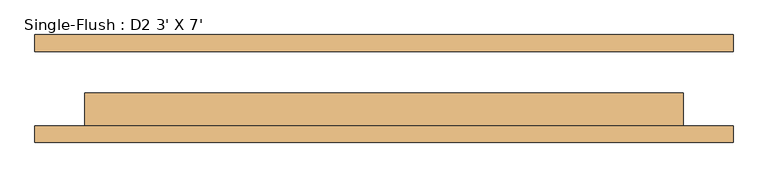
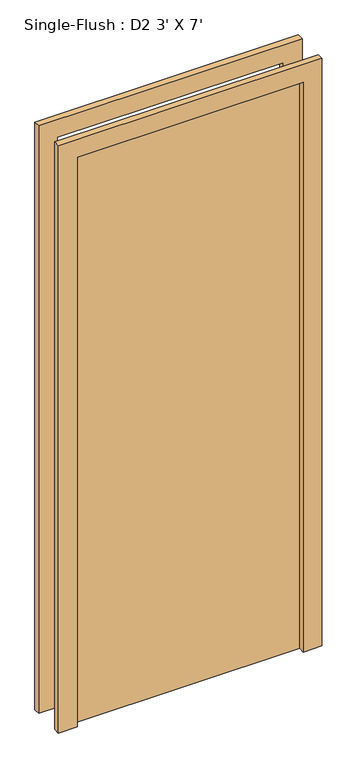
"""IFC4 building model written with IfcOpenShell, lengths in millimetres: door geometry, Single-Flush : D2 3' X 7'."""

from ifc_helpers import new_model, si_unit, frame, origin, origin_with_axes, place, context, project, spatial, polyline, outline, extrude, source, transform, mapped, element, save


def single_flush_d2_3_x_7_58d0fc15(model_context):
    return source(origin(), model_context, "Body", "SweptSolid", [
        extrude(outline(polyline([(2514.6, -533.4), (0.0, -533.4), (0.0, -457.2), (2438.4, -457.2), (2438.4, 457.2), (0.0, 457.2), (0.0, 533.4), (2514.6, 533.4), (2514.6, -533.4)])), frame((0.0, -82.55, 0.0), z_axis=(0.0, 1.0, 0.0), x_axis=(0.0, 0.0, 1.0)), (0.0, 0.0, 1.0), 25.4),
        extrude(outline(polyline([(2514.6, 533.4), (2514.6, -533.4), (0.0, -533.4), (0.0, -457.2), (2438.4, -457.2), (2438.4, 457.2), (0.0, 457.2), (0.0, 533.4), (2514.6, 533.4)])), frame((0.0, 57.15, 0.0), z_axis=(0.0, 1.0, 0.0), x_axis=(0.0, 0.0, 1.0)), (0.0, 0.0, 1.0), 25.4),
        extrude(outline(polyline([(457.2, -6.35), (457.2, -57.15), (-457.2, -57.15), (-457.2, -6.35), (457.2, -6.35)])), origin_with_axes(), (0.0, 0.0, 1.0), 2438.4),
    ])


if __name__ == "__main__":
    model = new_model("IFC4")
    model_context = context("Model", 3, world=origin())
    ifc_project = project(units=[si_unit("LENGTHUNIT", "METRE", prefix="MILLI")], contexts=[model_context])
    site = spatial("IfcSite", under=ifc_project)
    building = spatial("IfcBuilding", under=site)
    placement = place(None, origin())
    single_flush_d2_3_x_7_shape = single_flush_d2_3_x_7_58d0fc15(model_context)
    element("IfcDoor", 1, ObjectType="Single-Flush : D2 3' X 7'", at=placement, inside=building, context=model_context, shape_type="MappedRepresentation", body=[
        mapped(single_flush_d2_3_x_7_shape, transform((0.0, 0.0, 0.0), x_axis=(1.0, 0.0, 0.0), y_axis=(0.0, 1.0, 0.0), z_axis=(0.0, 0.0, 1.0))),
    ])
    save(model, "model.ifc")

# Revit data of these elements
# Type "Single-Flush : D2 3' X 7'"
#   Type Mark = "10"
#   Construction Type Id = "MDOOR"
#   Assembly Code = "C1020"
#   Analytic Construction = "Metal"
#   Thickness = 0' - 2"
#   Heat Transfer Coefficient (U) = 0.651978 BTU/(h·ft²·°F)
#   Height = 8' - 0"
#   Trim Projection Ext = 0' - 1"
#   Trim Projection Int = 0' - 1"
#   Trim Width = 0' - 3"
#   Width = 3' - 0"
#   Define Thermal Properties by = 1
#   Door Material = Door - Panel
#   Frame Material = Door - Frame
#   Visual Light Transmittance = 0
#   Solar Heat Gain Coefficient = 0
#   Function = (empty or 0)
#   Wall Closure = (empty or 0)
# Element 1 (IfcDoor, "Single-Flush : D2 3' X 7'")
#   Materials on its faces: "Door - Frame", "Door - Panel"
# Materials
#   "Door - Panel": class "Wood", colour RGB 210 159 95, transparency 0, Cost = 0
#   "Door - Frame": colour RGB 118 70 51, transparency 0, Cost = 0
